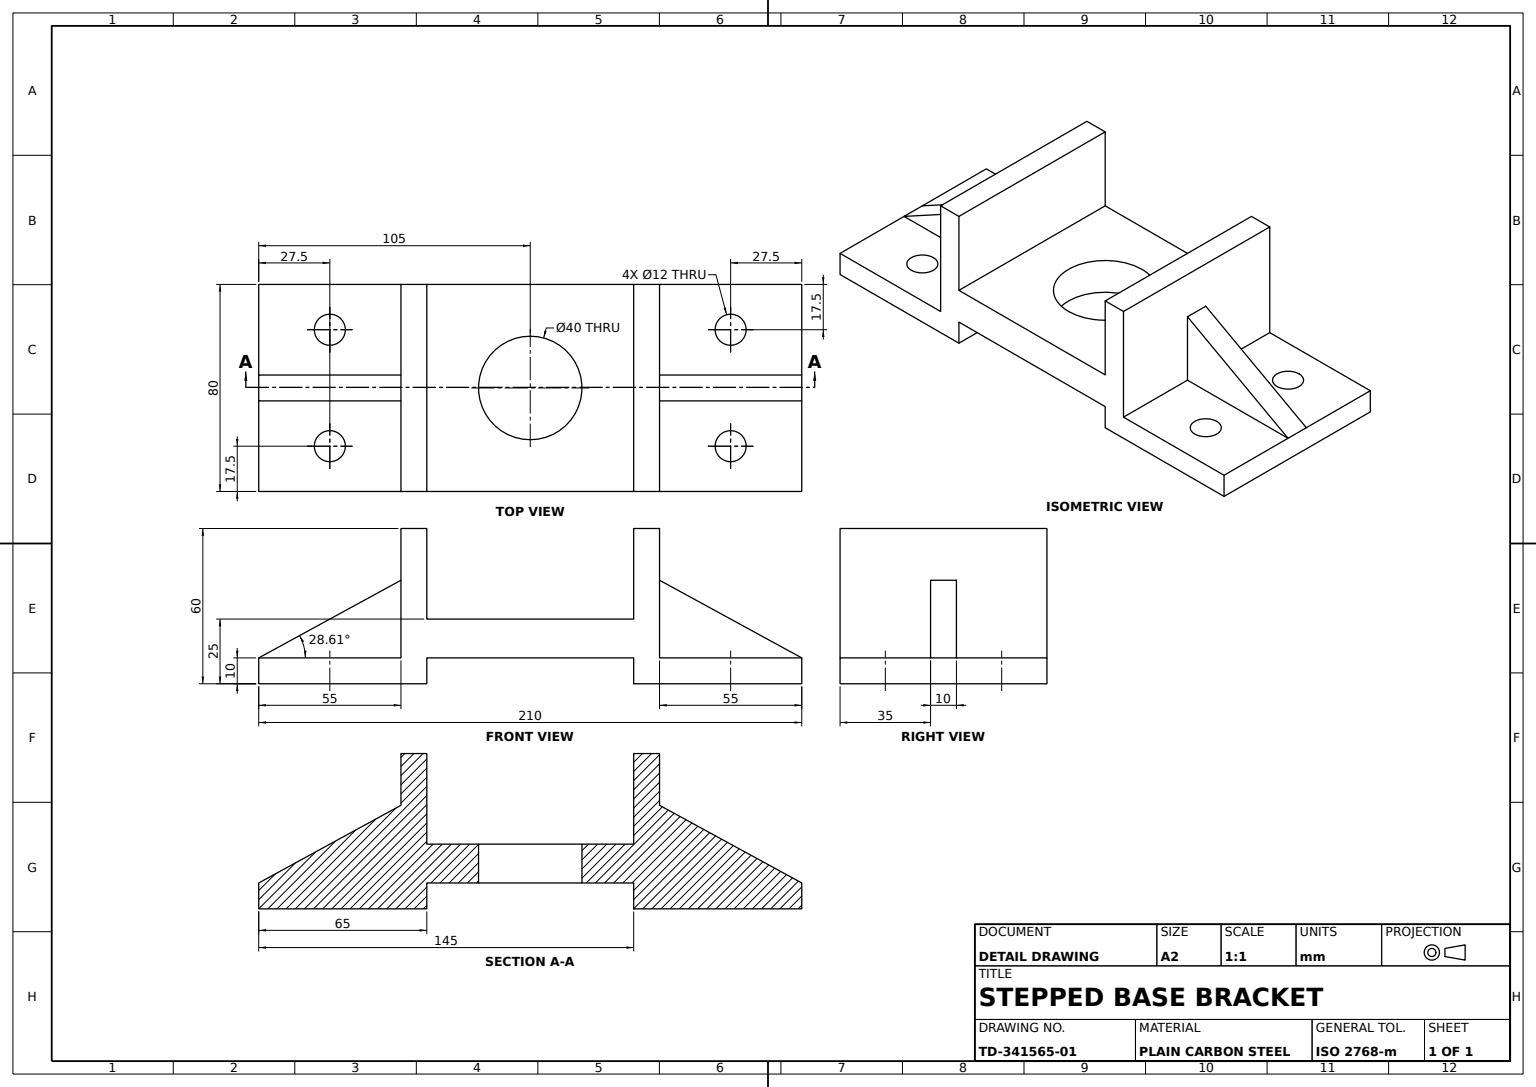
SolidWorks part; units mm, degrees
material "Plain Carbon Steel"
ref_plane "Front Plane" through (0, 0, 0) normal (0, 0, 1) x (1, 0, 0)
ref_plane "Top Plane" through (0, 0, 0) normal (0, 1, 0) x (1, 0, 0)
ref_plane "Right Plane" through (0, 0, 0) normal (1, 0, 0) x (0, 0, -1)
sketch "Base Profile Sketch" plane through (0, 0, 0) normal (0, 0, 1) x (1, 0, 0)
  line L0 (0, 0) -> (55, 0)
  line L1 (55, 0) -> (65, 0)
  line L2 (65, 0) -> (65, 10)
  line L3 (65, 10) -> (145, 10)
  line L4 (145, 10) -> (145, 0)
  line L5 (145, 0) -> (210, 0)
  line L6 (210, 0) -> (210, 10)
  line L7 (210, 10) -> (155, 10)
  line L8 (155, 10) -> (155, 60)
  line L9 (155, 60) -> (145, 60)
  line L10 (145, 60) -> (145, 25)
  line L11 (145, 25) -> (65, 25)
  line L12 (65, 25) -> (65, 60)
  line L13 (65, 60) -> (55, 60)
  line L14 (55, 60) -> (55, 10)
  line L15 (55, 10) -> (0, 10)
  line L16 (0, 10) -> (0, 0)
  dimension "D1" = 55
  dimension "D2" = 65
  dimension "D3" = 145
  dimension "D4" = 25
  dimension "D5" = 60
extrude "Base Body" add sketch "Base Profile Sketch" along normal blind 60
sketch "Center Bore Sketch" plane through (0, 25, 0) normal (0, 1, 0) x (1, 0, 0)
  line L0 (65, -60) -> (65, 0) construction
  line L1 (145, 0) -> (65, 0) construction
  circle A0 centre (105, -30) radius 20
  dimension "D1" = 40
  dimension "D2" = 40
  dimension "D3" = 30
extrude "Center Bore" cut sketch "Center Bore Sketch" against normal blind 15
sketch "Gusset 1 Sketch" plane through (0, 0, 60) normal (0, 0, 1) x (1, 0, 0)
  line L0 (155, 10) -> (155, 40)
  line L1 (155, 10) -> (155, 60) construction
  line L2 (155, 40) -> (210, 10)
  line L3 (210, 10) -> (155, 10)
  line L5 (0, 0) -> (65, 0) construction
  dimension "D1" = 40
extrude "Gusset 1 Blank" add sketch "Gusset 1 Sketch" against normal blind 40
sketch "Gusset 1 Trim A Sketch" plane through (0, 0, 60) normal (0, 0, 1) x (1, 0, 0)
  line L0 (155, 40) -> (155, 10)
  line L1 (155, 10) -> (210, 10)
  line L2 (210, 10) -> (155, 40)
extrude "Gusset 1 Trim A" cut sketch "Gusset 1 Trim A Sketch" against normal blind 25
sketch "Gusset 1 Trim B Sketch" plane through (0, 0, 20) normal (0, 0, -1) x (-1, 0, 0)
  line L0 (-210, 10) -> (-155, 10)
  line L1 (-155, 10) -> (-155, 40)
  line L2 (-155, 40) -> (-210, 10)
extrude "Gusset 1 Trim B" cut sketch "Gusset 1 Trim B Sketch" against normal blind 5
sketch "Gusset 2 Sketch" plane through (0, 0, 0) normal (0, 0, -1) x (-1, 0, 0)
  line L0 (-55, 10) -> (-55, 40)
  line L1 (-55, 60) -> (-55, 10) construction
  line L2 (-55, 40) -> (0, 10)
  line L3 (0, 10) -> (-55, 10)
  line L5 (-65, 60) -> (-55, 60) construction
  dimension "D1" = 20
extrude "Gusset 2 Blank" add sketch "Gusset 2 Sketch" against normal blind 35
sketch "Gusset 2 Trim Sketch" plane through (0, 0, 0) normal (0, 0, -1) x (-1, 0, 0)
  line L0 (-55, 40) -> (-55, 10)
  line L1 (-55, 10) -> (0, 10)
  line L2 (0, 10) -> (-55, 40)
extrude "Gusset 2 Trim" cut sketch "Gusset 2 Trim Sketch" against normal blind 25
sketch "Flange Extension 1 Sketch" plane through (0, 0, 60) normal (0, 0, 1) x (1, 0, 0)
  line L0 (0, 0) -> (0, 10)
  line L1 (0, 10) -> (55, 10)
  line L2 (55, 10) -> (55, 60)
  line L3 (55, 60) -> (65, 60)
  line L4 (65, 60) -> (65, 25)
  line L5 (65, 25) -> (145, 25)
  line L6 (145, 25) -> (145, 60)
  line L7 (145, 60) -> (155, 60)
  line L8 (155, 60) -> (155, 10)
  line L9 (155, 10) -> (210, 10)
  line L10 (210, 10) -> (210, 0)
  line L11 (210, 0) -> (145, 0)
  line L12 (145, 0) -> (145, 10)
  line L13 (145, 10) -> (65, 10)
  line L14 (65, 10) -> (65, 0)
  line L15 (65, 0) -> (0, 0)
extrude "Flange Extension 1" add sketch "Flange Extension 1 Sketch" along normal blind 10
sketch "Flange Extension 2 Sketch" plane through (0, 0, 0) normal (0, 0, -1) x (-1, 0, 0)
  line L0 (-210, 0) -> (-210, 10)
  line L1 (-210, 10) -> (-155, 10)
  line L2 (-155, 10) -> (-155, 60)
  line L3 (-155, 60) -> (-145, 60)
  line L4 (-145, 60) -> (-145, 25)
  line L5 (-145, 25) -> (-65, 25)
  line L6 (-65, 25) -> (-65, 60)
  line L7 (-65, 60) -> (-55, 60)
  line L8 (-55, 60) -> (-55, 10)
  line L9 (-55, 10) -> (0, 10)
  line L10 (0, 10) -> (0, 0)
  line L11 (0, 0) -> (-65, 0)
  line L12 (-65, 0) -> (-65, 10)
  line L13 (-65, 10) -> (-145, 10)
  line L14 (-145, 10) -> (-145, 0)
  line L15 (-145, 0) -> (-210, 0)
extrude "Flange Extension 2" add sketch "Flange Extension 2 Sketch" along normal blind 10
sketch "Mounting Holes Sketch" plane through (0, 10, 0) normal (0, 1, 0) x (1, 0, 0)
  line L0 (55, -70) -> (0, -70) construction
  line L1 (0, -70) -> (0, -35) construction
  line L2 (0, 10) -> (55, 10) construction
  line L4 (155, 10) -> (210, 10) construction
  line L5 (210, -70) -> (155, -70) construction
  line L6 (210, -70) -> (210, -35) construction
  line L7 (210, -25) -> (210, 10) construction
  circle A0 centre (27.5, -52.5) radius 6
  circle A1 centre (27.5, -7.5) radius 6
  circle A2 centre (182.5, -7.5) radius 6
  circle A3 centre (182.5, -52.5) radius 6
  dimension "D1" = 17.5
  dimension "D3" = 17.5
  dimension "D4" = 17.5
  dimension "D8" = 12
  dimension "D2" = 27.5
  dimension "D5" = 17.5
  dimension "D6" = 27.5
  dimension "D7" = 27.5
extrude "Mounting Holes 4x" cut sketch "Mounting Holes Sketch" against normal blind 10
